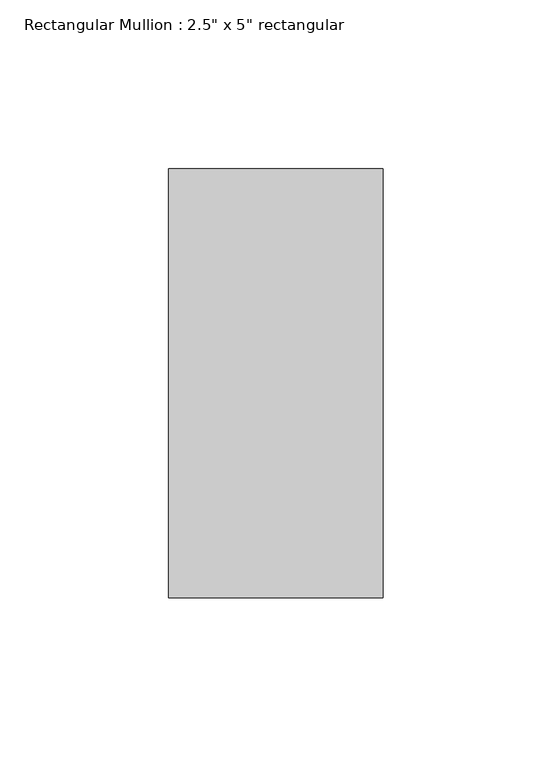
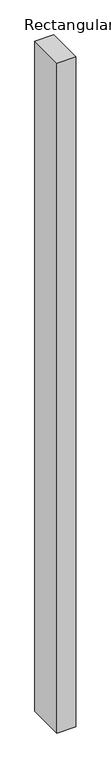
"""IFC4 building model written with IfcOpenShell, lengths in millimetres: member geometry."""

from ifc_helpers import new_model, si_unit, frame, origin, place, context, project, spatial, polyline, outline, extrude, source, transform, mapped, element, save


def member_0a963142(model_context):
    return source(origin(), model_context, "Body", "SweptSolid", [
        extrude(outline(polyline([(31.75, 63.5), (31.75, -63.5), (-31.75, -63.5), (-31.75, 63.5), (31.75, 63.5)])), frame((0.0, 0.0, -2364.5663272), z_axis=(0.0, 0.0, 1.0), x_axis=(1.0, 0.0, 0.0)), (0.0, 0.0, 1.0), 2364.5663272),
    ])


if __name__ == "__main__":
    model = new_model("IFC4")
    model_context = context("Model", 3, world=origin())
    ifc_project = project(units=[si_unit("LENGTHUNIT", "METRE", prefix="MILLI")], contexts=[model_context])
    site = spatial("IfcSite", under=ifc_project)
    building = spatial("IfcBuilding", under=site)
    placement = place(None, origin())
    member_shape = member_0a963142(model_context)
    element("IfcMember", 1, ObjectType="Rectangular Mullion : 2.5\" x 5\" rectangular", at=placement, inside=building, context=model_context, shape_type="MappedRepresentation", body=[
        mapped(member_shape, transform((0.0, 0.0, 0.0), x_axis=(1.0, 0.0, 0.0), y_axis=(0.0, 1.0, 0.0), z_axis=(0.0, 0.0, 1.0))),
    ])
    save(model, "model.ifc")

# Revit data of these elements
# Type "Rectangular Mullion : 2.5\" x 5\" rectangular"
#   built-in parameter 1007304 = 0.416667 (stored number, unit not read)
#   built-in parameter 1007301 = 0.104167 (stored number, unit not read)
#   built-in parameter 1007300 = 0.104167 (stored number, unit not read)
# Element 1 (IfcMember, "Rectangular Mullion : 2.5\" x 5\" rectangular")
#   Materials on its faces: "Aluminum"
# Materials
#   "Aluminum": class "Metal", colour RGB 247 247 247, transparency 0, Description = "Aluminum 6061", Cost = 0
